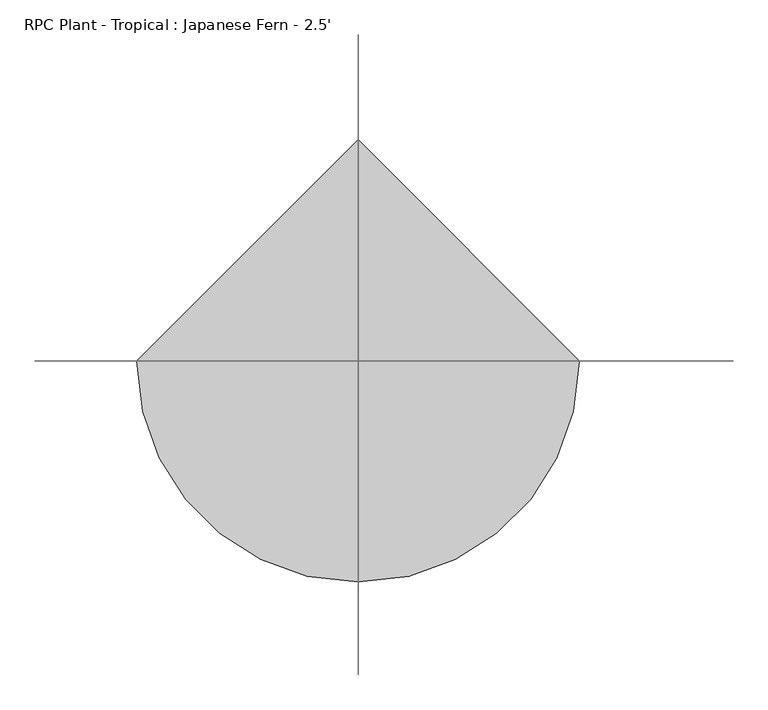
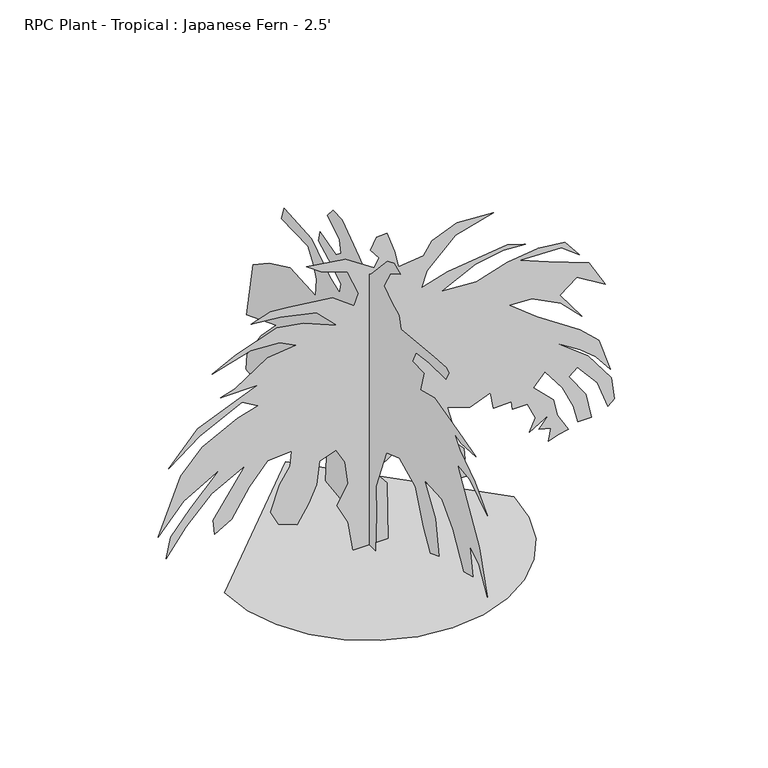
"""IFC4 building model written with IfcOpenShell, lengths in millimetres: geographic element geometry, RPC Plant - Tropical : Japanese Fern - 2.5'."""

from ifc_helpers import new_model, si_unit, origin, place, context, project, spatial, triangles, source, transform, mapped, element, save


def rpc_plant_tropical_japanese_fern_2_5_15da35ff(model_context):
    return source(origin(), model_context, "Body", "Tessellation", [
        triangles([(-544.3397392, 0.0, 3.74e-05), (-529.9491205, -124.7268799, 3.74e-05), (-488.967792, -239.2685712, 3.74e-05), (-424.6713169, -340.3433973, 3.74e-05), (-340.3433973, -424.6713169, 3.74e-05), (-239.2685712, -488.967792, 3.74e-05), (-124.7268799, -529.9491205, 3.74e-05), (2.38e-05, -544.3397392, 3.74e-05), (124.7268799, -529.9491205, 3.74e-05), (239.2685712, -488.967792, 3.74e-05), (340.3433973, -424.6713169, 3.74e-05), (424.6713169, -340.3433973, 3.74e-05), (488.967792, -239.2685712, 3.74e-05), (529.9491205, -124.7268799, 3.74e-05), (544.3397392, 4.76e-05, 3.74e-05), (-7.14e-05, 544.3397392, 3.74e-05), (-60.6368511, 3.66e-05, 5.8e-06), (-80.1399666, 3.85e-05, 117.6669093), (-121.4122839, 3.56e-05, 197.9743076), (-79.2865304, 2.93e-05, 272.8335282), (-91.1664011, 2.45e-05, 361.4936688), (-123.758834, 2.25e-05, 419.5913218), (-186.0204769, 2.65e-05, 397.3559784), (-197.60449, 3.23e-05, 308.4243791), (-228.9037605, 3.76e-05, 242.9233263), (-270.517445, 4.35e-05, 174.9944421), (-341.9275666, 4.5e-05, 202.0066014), (-372.0710029, 4.28e-05, 260.8768453), (-337.2254917, 3.55e-05, 357.3309142), (-297.557655, 3.02e-05, 416.9863209), (-291.7067222, 2.65e-05, 474.4634085), (-381.6982132, 3.08e-05, 468.5096294), (-452.3715157, 3.87e-05, 387.443502), (-517.7165096, 4.78e-05, 283.401942), (-581.6634785, 5.28e-05, 245.5950019), (-587.4506252, 4.96e-05, 304.4371951), (-466.1972342, 3.4e-05, 477.4057434), (-593.4897188, 4.35e-05, 410.8537374), (-688.5587706, 5.35e-05, 312.8585924), (-764.5961351, 6.28e-05, 213.2045371), (-747.9418465, 5.73e-05, 292.58007), (-673.3350632, 4.89e-05, 379.5589179), (-562.4448478, 3.71e-05, 496.2301758), (-698.7715919, 4.77e-05, 418.1770549), (-795.2914999, 5.84e-05, 308.4113711), (-709.6143167, 4.19e-05, 522.3535086), (-628.6554502, 3.33e-05, 608.1038341), (-495.8318716, 2.34e-05, 676.9519936), (-417.274857, 1.86e-05, 699.7672434), (-478.9459837, 1.92e-05, 735.2012724), (-638.2708517, 3.09e-05, 655.33965), (-754.9929422, 4.12e-05, 567.5045317), (-645.1106232, 2.92e-05, 688.188953), (-480.9698427, 1.8e-05, 756.9761061), (-420.1318411, 1.38e-05, 781.4779535), (-558.4093019, 1.99e-05, 781.1772451), (-505.0571443, 1.66e-05, 797.4088125), (-381.6982132, 6.4e-06, 877.6565306), (-275.8510403, 1e-06, 891.1123953), (-337.2254917, 1.8e-06, 922.128816), (-446.0601276, 6.2e-06, 928.7571905), (-590.7180493, 1.5e-05, 886.5525719), (-500.9118668, 8.4e-06, 932.711455), (-346.6978786, -1.5e-06, 985.7181759), (-246.5581698, -4.9e-06, 968.8362848), (-120.1187128, -7.3e-06, 915.4272629), (-197.5866132, -8.5e-06, 993.0211458), (-334.5526171, -4.2e-06, 1022.1965452), (-443.9590568, -1e-07, 1033.3075676), (-371.5829513, -4.8e-06, 1058.4677324), (-304.0141286, -7.4e-06, 1052.3433243), (-137.1533561, -1.34e-05, 1031.3690231), (-57.050374, -1.33e-05, 971.0471237), (-39.2614525, -1.68e-05, 1015.5194092), (-81.3868019, -2.08e-05, 1113.9168915), (-181.4415776, -1.85e-05, 1149.1842882), (-234.9396021, -1.85e-05, 1188.9626741), (-88.9303912, -2.37e-05, 1168.3785381), (18.5524264, -2.41e-05, 1095.5720083), (37.0429969, -2.69e-05, 1129.7461578), (5.2108148, -2.8e-05, 1171.1745157), (28.206327, -3.15e-05, 1213.3507204), (66.3967512, -3.34e-05, 1216.8985416), (95.4323744, -2.97e-05, 1134.3953653), (109.6250673, -2.64e-05, 1068.9528482), (203.9536664, -3.12e-05, 1078.771435), (236.466453, -3.54e-05, 1126.7022303), (329.8587175, -4.19e-05, 1166.7244967), (467.7212328, -4.74e-05, 1157.8324522), (324.5356776, -3.88e-05, 1117.895573), (217.8866641, -2.8e-05, 1014.9504759), (198.0121141, -2.34e-05, 952.7469326), (294.2804568, -2.95e-05, 984.3892599), (521.0896322, -4.1e-05, 1011.073387), (587.978936, -4.27e-05, 991.0094954), (505.1059422, -3.94e-05, 995.5002096), (399.5326624, -3.36e-05, 975.7126093), (273.2000938, -2.43e-05, 913.1148314), (403.613736, -2.96e-05, 905.8443449), (521.0449039, -3.68e-05, 941.2174038), (636.7184029, -4.29e-05, 957.7050602), (736.2903774, -4.65e-05, 945.736532), (792.3695126, -4.49e-05, 877.6565306), (724.7202261, -4.5e-05, 928.8303692), (568.0694318, -3.84e-05, 933.2763187), (672.294647, -4.04e-05, 890.9985941), (826.9337545, -4.37e-05, 832.7209013), (890.0557737, -4.01e-05, 725.5370367), (782.8881872, -3.93e-05, 791.064941), (719.0752945, -3.36e-05, 741.890617), (801.2655539, -3.04e-05, 628.6107582), (721.2129547, -3.17e-05, 708.6633574), (612.9521936, -3.03e-05, 764.3888803), (527.9903011, -2.69e-05, 769.4972895), (632.2683838, -2.65e-05, 686.4251799), (793.0644556, -2.71e-05, 578.9975075), (865.700211, -2.62e-05, 510.7467679), (908.1283625, -2.03e-05, 379.8133355), (854.2925497, -2.21e-05, 449.4413893), (796.1612143, -2.24e-05, 497.1405127), (704.3107887, -2.18e-05, 554.6663618), (823.4996618, -2.16e-05, 464.0636436), (912.9522686, -1.84e-05, 345.5770168), (922.6449183, -1.37e-05, 258.5095661), (899.1021692, -1.14e-05, 237.2556853), (859.0799755, -1.6e-05, 343.989214), (783.4774681, -1.8e-05, 432.9334216), (751.2743465, -1.5e-05, 406.5540361), (816.9241184, -1.23e-05, 312.8423507), (836.841798, -7.3e-06, 215.0195244), (786.73272, -5.1e-06, 213.7633329), (769.8142759, -8.4e-06, 282.1055277), (727.6259354, -1.18e-05, 370.6417296), (661.6551075, -1.41e-05, 456.1998067), (618.4020063, -9.3e-06, 408.9192624), (694.5328245, -8.3e-06, 335.0947351), (709.0900755, -4.8e-06, 266.5709018), (749.8438379, -2.5e-06, 198.3425082), (714.2147627, -4e-07, 189.2631387), (674.4079628, 2e-06, 176.9471935), (684.8076914, -1.2e-06, 223.8424597), (639.2665758, 0.0, 236.2864131), (676.7406693, -4.3e-06, 281.727989), (603.544047, 1.5e-06, 237.7482243), (625.9610653, -2.4e-06, 286.6450035), (596.7449707, -4.9e-06, 350.2225545), (538.6542214, -2.4e-06, 350.5367068), (535.8053401, -4.1e-06, 381.2816689), (467.7212328, -1e-06, 379.5670569), (457.3296069, -4.4e-06, 444.4020166), (378.7778246, 8e-07, 415.1452995), (294.2804568, 2.9e-06, 441.8294992), (320.963839, 7.5e-06, 343.989214), (319.0691872, 1.03e-05, 299.4908946), (356.5416819, 1.1e-05, 259.4918281), (360.9889031, 1.35e-05, 215.0195244), (333.6878079, 1.59e-05, 194.5207211), (380.5505362, 1.68e-05, 144.7168661), (291.2617094, 2.05e-05, 148.5459565), (306.4253005, 1.59e-05, 213.3532926), (264.7327509, 1.6e-05, 243.5487787), (277.7412047, 1.31e-05, 282.1624283), (174.4791392, 1.83e-05, 271.3700819), (151.9694667, 1.7e-05, 308.4113711), (232.0196314, 1.09e-05, 352.8836929), (133.3165446, 1.49e-05, 357.9791305), (18.6823523, 2.43e-05, 283.5502796), (67.4720852, 2.58e-05, 223.9139852), (71.9193156, 2.91e-05, 0.0), (0.0033921, 42.710161, 5.7e-06), (0.0034005, 35.5325332, 200.3769407), (0.0034034, 96.2715946, 206.1250637), (0.0034015, 191.0456062, 68.7396451), (0.0034062, 284.7930453, 81.7968604), (0.0034102, 277.5331324, 181.0168761), (0.003414, 220.105206, 323.8744534), (0.0034079, 218.5186204, 404.0948839), (0.0034107, 267.8526913, 420.5991817), (0.0034193, 362.2333039, 304.4371951), (0.0034197, 461.3691859, 213.545105), (0.0034221, 505.0124522, 224.5768262), (0.0034252, 495.8278384, 304.1027133), (0.0034293, 554.6176003, 340.0199069), (0.0034309, 655.0552197, 275.3970891), (0.0034307, 725.2322588, 200.3769407), (0.0034346, 802.6757875, 212.4770924), (0.003437, 795.4134401, 275.3970891), (0.0034291, 705.8754461, 403.6571926), (0.0034293, 606.2303292, 507.0485198), (0.0034344, 797.8355307, 432.6977165), (0.0034424, 755.5740841, 656.8229897), (0.0034409, 652.6330564, 725.5167618), (0.0034377, 517.1150202, 788.4395926), (0.00343, 348.2267461, 780.7179708), (0.0034327, 342.8732574, 848.9362633), (0.0034356, 363.0668286, 894.5626934), (0.0034395, 398.9409471, 946.9801334), (0.0034472, 572.7714704, 950.5767889), (0.0034487, 555.832715, 1001.3970154), (0.0034404, 376.6129495, 990.0097017), (0.0034318, 258.0946205, 912.0622793), (0.0034278, 191.5223032, 886.5119493), (0.0034293, 184.713907, 927.2859867), (0.0034349, 265.4329807, 974.7778553), (0.0034392, 330.7730876, 1008.6594355), (0.003431, 318.6729541, 1052.2173145), (0.0034253, 214.8085998, 1024.0294275), (0.003425, 183.1529194, 1049.7992208), (0.0034274, 192.6842053, 1096.2385374), (0.0034331, 272.6929118, 1146.5995623), (0.0034334, 236.3928928, 1187.7394203), (0.0034307, 178.3126988, 1185.3172571), (0.0034224, 66.7039908, 1105.7848297), (0.0034184, 17.1942789, 1065.5513117), (0.003418, -16.1882776, 1088.8014187), (0.0034183, -119.3477751, 1199.8378824), (0.0034173, -162.9077162, 1219.1987646), (0.0034146, -204.0479558, 1199.8378824), (0.0034158, -139.4316328, 1162.2784744), (0.0034145, -97.2684905, 1089.5369843), (0.0034106, -148.0432438, 1052.1522749), (0.0034076, -194.8873049, 1030.8040867), (0.0034146, -207.6059871, 984.3363562), (0.0033965, -424.2689795, 1006.2372723), (0.0033933, -504.1305656, 1011.0774565), (0.003392, -521.069321, 998.9789944), (0.0034008, -501.7084388, 962.6793932), (0.0034056, -389.8375783, 961.5292454), (0.0034088, -306.9511768, 950.1215841), (0.0034077, -282.5550097, 901.252038), (0.0034044, -357.3455209, 899.8947081), (0.0034019, -334.4250086, 819.6998211), (0.0033989, -426.6870732, 844.1000759), (0.0033901, -586.4752487, 803.0862276), (0.003384, -695.3090853, 771.496804), (0.003388, -600.4797718, 768.0952675), (0.0033904, -557.4705148, 779.815773), (0.0033869, -592.0185513, 735.5223284), (0.0033798, -689.2821276, 670.0472551), (0.0033725, -772.7484718, 585.158505), (0.0033807, -656.6564301, 658.0828691), (0.0033847, -576.6037946, 668.567985), (0.0033773, -637.5230776, 561.9043284), (0.0033678, -719.5101517, 425.4353328), (0.0033678, -770.9359371, 259.4918281), (0.0033648, -717.0879885, 355.2570582), (0.003369, -656.7580227, 391.1246727), (0.0033635, -677.4762348, 284.2935845), (0.0033748, -619.7309223, 268.3862888), (0.0033739, -547.688481, 393.9771875), (0.0033805, -474.3414682, 469.9523466), (0.0033857, -361.7931782, 477.4057434), (0.0033777, -433.9494206, 367.3571918), (0.0033804, -454.9399635, 231.302742), (0.0033818, -398.9913437, 208.0538341), (0.0033872, -354.8742328, 286.9790674), (0.0033856, -301.0925228, 414.5844689), (0.0033923, -198.3819317, 464.1611667), (0.0033947, -112.1146774, 433.8315499), (0.0033996, -43.9972282, 259.7771304), (0.0033947, -48.6976453, 151.3643437), (0.0033884, -41.1219494, 3.89e-05)], [[15, 16, 1], [14, 15, 1], [14, 1, 2], [13, 14, 2], [13, 2, 3], [13, 3, 4], [12, 13, 4], [11, 12, 4], [11, 4, 5], [11, 5, 6], [11, 6, 7], [11, 7, 8], [11, 8, 9], [11, 9, 10], [110, 111, 112], [51, 52, 53], [61, 62, 63], [102, 103, 104], [94, 95, 96], [55, 56, 57], [88, 89, 90], [44, 45, 46], [117, 118, 119], [61, 63, 64], [68, 69, 70], [39, 40, 41], [107, 108, 109], [76, 77, 78], [39, 41, 42], [75, 76, 78], [38, 39, 42], [38, 42, 43], [60, 61, 64], [143, 144, 145], [93, 94, 96], [93, 96, 97], [93, 97, 98], [68, 70, 71], [37, 38, 43], [55, 57, 58], [157, 158, 159], [157, 159, 160], [75, 78, 79], [92, 93, 98], [74, 75, 79], [67, 68, 71], [67, 71, 72], [110, 112, 113], [139, 140, 141], [87, 88, 90], [87, 90, 91], [86, 87, 91], [117, 119, 120], [116, 117, 120], [116, 120, 121], [115, 116, 121], [101, 102, 104], [101, 104, 105], [100, 101, 105], [106, 107, 109], [34, 35, 36], [141, 142, 143], [43, 44, 46], [43, 46, 47], [124, 125, 126], [123, 124, 126], [122, 123, 126], [122, 126, 127], [34, 36, 37], [33, 34, 37], [32, 33, 37], [60, 64, 65], [59, 60, 65], [137, 138, 139], [137, 139, 141], [137, 141, 143], [136, 137, 143], [121, 122, 127], [50, 51, 53], [50, 53, 54], [66, 67, 72], [66, 72, 73], [106, 109, 110], [106, 110, 113], [129, 130, 131], [129, 131, 132], [129, 132, 133], [128, 129, 133], [128, 133, 134], [43, 47, 48], [37, 43, 48], [105, 106, 113], [105, 113, 114], [100, 105, 114], [99, 100, 114], [59, 65, 66], [163, 164, 165], [162, 163, 165], [168, 169, 17], [168, 17, 18], [168, 18, 19], [168, 19, 20], [167, 168, 20], [167, 20, 21], [146, 147, 148], [121, 127, 128], [121, 128, 134], [85, 86, 91], [148, 149, 150], [37, 48, 49], [32, 37, 49], [31, 32, 49], [85, 91, 92], [25, 26, 27], [25, 27, 28], [25, 28, 29], [24, 25, 29], [24, 29, 30], [23, 24, 30], [23, 30, 31], [136, 143, 145], [135, 136, 145], [135, 145, 146], [135, 146, 148], [82, 83, 84], [81, 82, 84], [80, 81, 84], [80, 84, 85], [79, 80, 85], [50, 54, 55], [49, 50, 55], [160, 161, 162], [156, 157, 160], [155, 156, 160], [155, 160, 162], [154, 155, 162], [154, 162, 165], [153, 154, 165], [152, 153, 165], [74, 79, 85], [74, 85, 92], [73, 74, 92], [166, 167, 21], [55, 58, 59], [166, 21, 22], [152, 165, 166], [135, 148, 150], [134, 135, 150], [121, 134, 150], [115, 121, 150], [114, 115, 150], [114, 150, 151], [114, 151, 152], [99, 114, 152], [98, 99, 152], [98, 152, 166], [98, 166, 22], [92, 98, 22], [73, 92, 22], [66, 73, 22], [59, 66, 22], [55, 59, 22], [49, 55, 22], [31, 49, 22], [23, 31, 22], [244, 245, 246], [239, 240, 241], [234, 235, 236], [234, 236, 237], [233, 234, 237], [238, 239, 241], [238, 241, 242], [217, 218, 219], [216, 217, 219], [189, 190, 191], [244, 246, 247], [215, 216, 219], [215, 219, 220], [197, 198, 199], [197, 199, 200], [230, 231, 232], [189, 191, 192], [209, 210, 211], [209, 211, 212], [209, 212, 213], [208, 209, 213], [197, 200, 201], [196, 197, 201], [195, 196, 201], [243, 244, 247], [262, 170, 171], [261, 262, 171], [260, 261, 171], [205, 206, 207], [204, 205, 207], [203, 204, 207], [185, 186, 187], [184, 185, 187], [184, 187, 188], [183, 184, 188], [183, 188, 189], [173, 174, 175], [172, 173, 175], [172, 175, 176], [247, 248, 249], [247, 249, 250], [243, 247, 250], [243, 250, 251], [242, 243, 251], [254, 255, 256], [253, 254, 256], [253, 256, 257], [252, 253, 257], [225, 226, 227], [224, 225, 227], [224, 227, 228], [223, 224, 228], [223, 228, 229], [223, 229, 230], [180, 181, 182], [179, 180, 182], [189, 192, 193], [189, 193, 194], [252, 257, 258], [203, 207, 208], [242, 251, 252], [208, 213, 214], [203, 208, 214], [183, 189, 194], [182, 183, 194], [179, 182, 194], [178, 179, 194], [177, 178, 194], [195, 201, 202], [194, 195, 202], [177, 194, 202], [237, 238, 242], [237, 242, 252], [233, 237, 252], [232, 233, 252], [232, 252, 258], [230, 232, 258], [230, 258, 259], [223, 230, 259], [221, 222, 223], [221, 223, 259], [220, 221, 259], [215, 220, 259], [214, 215, 259], [203, 214, 259], [202, 203, 259], [177, 202, 259], [177, 259, 260], [176, 177, 260], [172, 176, 260], [172, 260, 171]], closed=False),
    ])


if __name__ == "__main__":
    model = new_model("IFC4")
    model_context = context("Model", 3, world=origin())
    ifc_project = project(units=[si_unit("LENGTHUNIT", "METRE", prefix="MILLI")], contexts=[model_context])
    site = spatial("IfcSite", under=ifc_project)
    building = spatial("IfcBuilding", under=site)
    placement = place(None, origin())
    rpc_plant_tropical_japanese_fern_2_5_shape = rpc_plant_tropical_japanese_fern_2_5_15da35ff(model_context)
    element("IfcGeographicElement", 1, ObjectType="RPC Plant - Tropical : Japanese Fern - 2.5'", at=placement, inside=building, context=model_context, shape_type="MappedRepresentation", body=[
        mapped(rpc_plant_tropical_japanese_fern_2_5_shape, transform((0.0, 0.0, 0.0), x_axis=(1.0, 0.0, 0.0), y_axis=(0.0, 1.0, 0.0), z_axis=(0.0, 0.0, 1.0))),
    ])
    save(model, "model.ifc")

# Revit data of these elements
# Type "RPC Plant - Tropical : Japanese Fern - 2.5'"
#   built-in parameter 1005198 = "{2, 15},{39, RPC-16-G1GK-JAPX-7J4P-Q000-ST1L-LVER-AU},{1, 0},{1, 0},{2, 35},{1, 8},{5, Color},{1, 0},{1, 0},{3, 0.8},{3, 0.8},{3, 0.8},{1, 8},{7, BBoxMin},{1, 0},{1, 0},{1, 0},{1, 0},{1, 0},{1, 8},{7, BBoxMax},{1, 0},{1, 0},{1, 0},{1, 0},{1, 0},{2, 11},{9, RPCTypeId},{1, 0},{1, 0},{39, RPC-16-G1GK-JAPX-7J4P-Q000-ST1L-LVER-AU},{1, 6},{14, RPCPlantHeight},{1, 0},{1, 0},{3, 2.5},{2, 11},{7, keyword},{1, 0},{1, 0},{53, :Geometry:RPC:Japanese Fern:plant:small:japanese fern},{2, 11},{8, category},{1, 0},{1, 0},{17, :Shrubs [General]},{2, 11},{12, LocalizedUID},{1, 0},{1, 0},{13, Japanese Fern},{2, 14},{6, Height},{1, 0},{1, 0},{3, 2.5},{1, 2},{16, Cast Reflections},{1, 0},{1, 0},{1, 0},{1, 2},{12, Cast Shadows},{1, 0},{1, 0},{1, 1},{1, 2},{9, Lock View},{1, 0},{1, 0},{1, 0},{1, 4},{5, ViewC},{1, 0},{1, 0},{1, 0},{2, 11},{20, AdvancedUIDefinition},{1, 0},{1, 0},{0, },{2, 11},{10, AssetLibID},{1, 0},{1, 0},{36, 4D3F6E72-3F99-4203-98E9-AF80B3C7A7A4},{2, 11},{10, BaseSchema},{1, 0},{1, 0},{9, RPCSchema},{2, 11},{12, ExchangeGUID},{1, 0},{1, 0},{0, },{1, 2},{6, Hidden},{1, 0},{1, 0},{1, 0},{1, 4},{11, RPCCategory},{1, 0},{1, 0},{1, 0},{2, 11},{8, RPCImage},{1, 0},{1, 0},{0, },{1, 4},{13, SchemaVersion},{1, 0},{1, 0},{1, 4},{2, 11},{12, UIDefinition},{1, 0},{1, 0},{0, },{2, 11},{6, UIName},{1, 0},{1, 0},{39, RPC-16-G1GK-JAPX-7J4P-Q000-ST1L-LVER-AU},{2, 11},{11, VersionGUID},{1, 0},{1, 0},{9, RPCSchema},{2, 11},{9, assettype},{1, 0},{1, 0},{11, RPCGeometry},{2, 11},{11, description},{1, 0},{1, 0},{0, },{2, 11},{9, localname},{1, 0},{1, 0},{3, RPC},{2, 11},{9, localtype},{1, 0},{1, 0},{3, RPC},{1, 4},{8, revision},{1, 0},{1, 0},{1, 1},{2, 11},{9, thumbnail},{1, 0},{1, 0},{0, },{1, 4},{7, version},{1, 0},{1, 0},{1, 1},{1, 2},{20, RPC_Cast Reflections},{1, 0},{1, 0},{1, 1},{1, 2},{16, RPC_Cast Shadows},{1, 0},{1, 0},{1, 1},{1, 2},{13, RPC_Lock View},{1, 0},{1, 0},{1, 0},{1, 4},{9, RPC_ViewC},{1, 0},{1, 0},{1, 0},{21, assetlibrary_base.fbx},{1, 5},"
#   built-in parameter 1005195 = "RPC-16-G1GK-JAPX-7J4P-Q000-ST1L-LVER-AU"
#   Type Comments = "Japanese Fern"
#   Assembly Code = "G2050500"
#   Height = 4' - 0"
#   Default Elevation = 0
